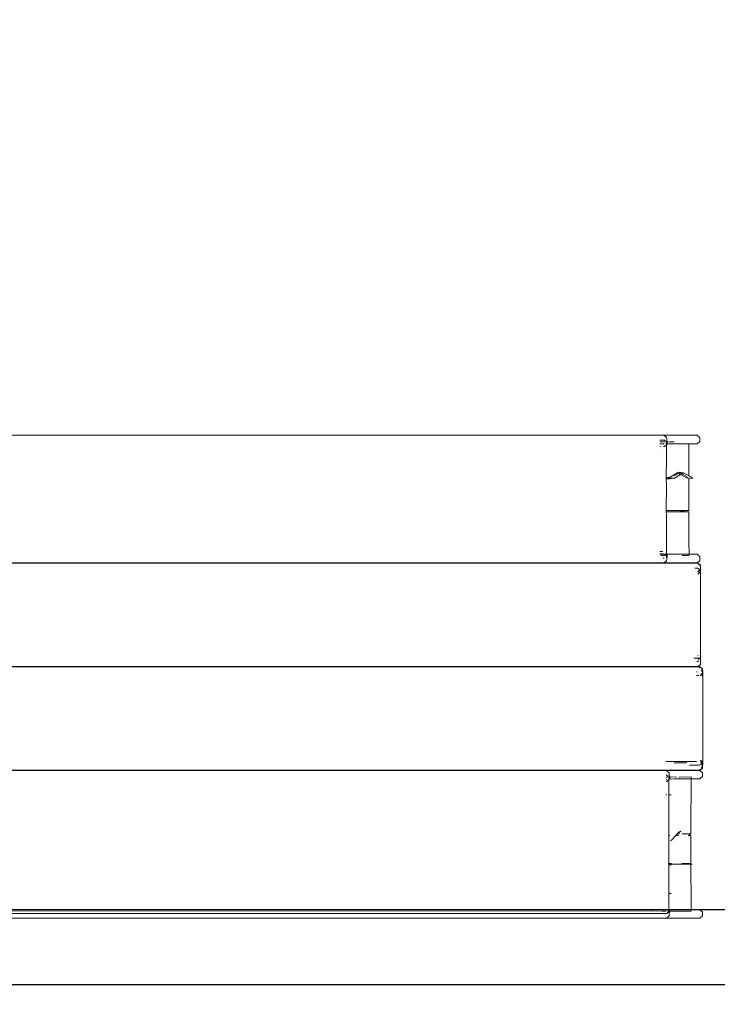
# Model space of a CAD drawing. Units: millimetres. Extents: x 7894 to 8038, y 6851 to 6951.
# Tile 4 of 49: x 7949.503 to 7954.151, y 6864.931 to 6871.489. Entities that reach past the tile are written whole.
import ezdxf

# ---------------------------------------------------------------- set-up
doc = ezdxf.new("R2010")
doc.units = ezdxf.units.MM
for name, color, linetype, lineweight in [('A-ANNO-DIMS', 2, 'Continuous', 18), ('A-FURN-BOOK', 8, 'Continuous', 13), ('A-FURN-CASE', 7, 'Continuous', 30)]:
    doc.layers.add(name, color=color, linetype=linetype, lineweight=lineweight)
doc.styles.get("Standard").update_dxf_attribs({"font": 'arial.ttf'})
doc.dimstyles.new('ISO-25', dxfattribs={"dimtxt": 1, "dimasz": 1, "dimexe": 1.25, "dimexo": 0.625, "dimtad": 1, "dimdec": 0, "dimlunit": 4, "dimtxsty": 'Standard', "dimcen": 2.5, "dimclrt": 1, "dimadec": 0, "dimazin": 0, "dimtfac": 1, "dimtdec": 0, "dimtmove": 0, "dimatfit": 3, "dimfxl": 1, "dimarcsym": 0})

# ---------------------------------------------------------------- blocks, each defined once
blk = doc.blocks.new('*D36')
at = {"layer": 'A-ANNO-DIMS', "color": 0, "lineweight": -2, "transparency": 16777216}
for p, q in [((7980.8359, 6877.9586), (7980.8359, 6858.5122)), ((7944.4866, 6864.4359), (7944.4866, 6858.5122)), ((7945.4866, 6859.7622), (7979.8359, 6859.7622))]:
    blk.add_line(p, q, dxfattribs=at)
at = {"layer": 'A-ANNO-DIMS', "color": 0, "transparency": 16777216}
for points in [[(7945.4866, 6859.9288), (7945.4866, 6859.5955), (7944.4866, 6859.7622)], [(7979.8359, 6859.9288), (7979.8359, 6859.5955), (7980.8359, 6859.7622)]]:
    blk.add_solid(points, dxfattribs=at)
at = {"layer": 'Defpoints', "color": 0, "transparency": 16777216}
for p in [(7980.8359, 6878.5836), (7944.4866, 6865.0609), (7980.8359, 6859.7622)]:
    blk.add_point(p, dxfattribs=at)
at = {"layer": 'A-ANNO-DIMS', "color": 1, "transparency": 16777216, "insert": (7962.6613, 6860.9046), "char_height": 1, "attachment_point": 5}
blk.add_mtext('3\'-0 1/2"', dxfattribs=at)
blk = doc.blocks.new('*D37')
at = {"layer": 'A-ANNO-DIMS', "color": 0, "lineweight": -2, "transparency": 16777216}
for p, q in [((7954.9197, 6887.9028), (7941.3891, 6887.9028)), ((7942.6391, 6862.6097), (7942.6391, 6886.9028)), ((7953.6228, 6861.6097), (7941.3891, 6861.6097))]:
    blk.add_line(p, q, dxfattribs=at)
at = {"layer": 'A-ANNO-DIMS', "color": 0, "transparency": 16777216}
for points in [[(7942.4724, 6886.9028), (7942.8057, 6886.9028), (7942.6391, 6887.9028)], [(7942.4724, 6862.6097), (7942.8057, 6862.6097), (7942.6391, 6861.6097)]]:
    blk.add_solid(points, dxfattribs=at)
at = {"layer": 'Defpoints', "color": 0, "transparency": 16777216}
for p in [(7942.6391, 6887.9028), (7955.5447, 6887.9028), (7954.2478, 6861.6097)]:
    blk.add_point(p, dxfattribs=at)
at = {"layer": 'A-ANNO-DIMS', "color": 1, "transparency": 16777216, "insert": (7941.497, 6874.7562), "char_height": 1, "attachment_point": 5, "rotation": 90}
blk.add_mtext('2\'-2 1/2"', dxfattribs=at)

msp = doc.modelspace()

# ---------------------------------------------------------------- linework, layer by layer
at = {"layer": 'A-FURN-BOOK'}
for p, q in [((7953.7957, 6868.7211), (7945.1072, 6868.7211)), ((7953.7988, 6868.6885), (7953.7677, 6868.6885)), ((7953.8027, 6868.7151), (7953.7957, 6868.7211)), ((7954.0176, 6868.7211), (7953.7957, 6868.7211)), ((7953.8072, 6868.6808), (7953.7988, 6868.6885)), ((7953.8027, 6868.7151), (7953.8123, 6868.7081)), ((7953.8123, 6868.7069), (7953.8123, 6868.7081)), ((7953.8133, 6868.706), (7953.8123, 6868.7069)), ((7953.8131, 6868.677), (7953.8143, 6868.693)), ((7953.8143, 6868.693), (7953.8133, 6868.706)), ((7953.8158, 6868.6777), (7953.8143, 6868.693)), ((7954.0176, 6868.7211), (7954.0351, 6868.705)), ((7954.0351, 6868.705), (7954.0351, 6868.6797)), ((7953.7697, 6868.6769), (7953.7676, 6868.6775)), ((7953.7676, 6868.6636), (7953.7935, 6868.6636)), ((7953.7721, 6868.6458), (7953.7676, 6868.6458)), ((7953.8046, 6868.6775), (7953.7697, 6868.6769)), ((7953.7961, 6868.6612), (7953.7935, 6868.6612)), ((7953.7988, 6868.6458), (7953.7935, 6868.6458)), ((7953.7973, 6868.6621), (7953.7961, 6868.6612)), ((7953.8126, 6868.6585), (7953.7988, 6868.6458)), ((7953.8114, 6868.6769), (7953.8131, 6868.677)), ((7953.8132, 6868.6753), (7953.8114, 6868.6769)), ((7953.8132, 6868.6742), (7953.8114, 6868.6729)), ((7953.8114, 6868.6636), (7953.8132, 6868.6742)), ((7953.8126, 6868.6618), (7953.8114, 6868.6636)), ((7953.8127, 6868.6636), (7953.8114, 6868.6636)), ((7953.8124, 6868.5618), (7953.8125, 6868.6434)), ((7953.8125, 6868.6434), (7953.8126, 6868.6585)), ((7953.8163, 6868.6619), (7953.8126, 6868.6585)), ((7953.8126, 6868.6585), (7953.8126, 6868.6618)), ((7953.8168, 6868.6626), (7953.8127, 6868.6636)), ((7953.8131, 6868.677), (7953.8158, 6868.6777)), ((7953.8132, 6868.6753), (7953.8131, 6868.677)), ((7953.8163, 6868.6724), (7953.8132, 6868.6753)), ((7953.8132, 6868.6742), (7953.8132, 6868.6753)), ((7953.8192, 6868.6797), (7953.8158, 6868.6777)), ((7953.8158, 6868.6777), (7953.8187, 6868.6773)), ((7953.8163, 6868.6724), (7953.8158, 6868.6777)), ((7953.8163, 6868.6619), (7953.8168, 6868.6626)), ((7953.8168, 6868.6626), (7953.8172, 6868.6668)), ((7953.8168, 6868.6626), (7953.823, 6868.6636)), ((7953.8172, 6868.6668), (7953.8182, 6868.6753)), ((7953.8182, 6868.6753), (7953.8187, 6868.6773)), ((7953.8187, 6868.6773), (7953.8192, 6868.6797)), ((7953.8187, 6868.6773), (7953.8224, 6868.6775)), ((7953.823, 6868.6636), (7953.9622, 6868.6636)), ((7953.8317, 6868.6771), (7953.828, 6868.6775)), ((7953.8639, 6868.6775), (7953.8317, 6868.6771)), ((7953.9622, 6868.6636), (7953.9615, 6868.5883)), ((7953.9622, 6868.6636), (7954.0176, 6868.6636)), ((7954.0351, 6868.6797), (7954.0176, 6868.6636)), ((7953.769, 6868.5883), (7953.7676, 6868.5883)), ((7953.8113, 6868.4406), (7953.8124, 6868.5618)), ((7953.9615, 6868.5883), (7953.9608, 6868.4903)), ((7953.9608, 6868.4903), (7953.9607, 6868.4519)), ((7953.8123, 6868.4394), (7953.8113, 6868.4406)), ((7953.8113, 6868.4394), (7953.8113, 6868.4406)), ((7953.8113, 6868.4394), (7953.8123, 6868.4394)), ((7953.8113, 6868.4363), (7953.8113, 6868.4394)), ((7953.8113, 6868.4363), (7953.8123, 6868.4363)), ((7953.8113, 6868.4348), (7953.8113, 6868.4363)), ((7953.8113, 6868.4348), (7953.8373, 6868.435)), ((7953.8113, 6868.432), (7953.8113, 6868.4348)), ((7953.8113, 6868.432), (7953.8123, 6868.4308)), ((7953.8113, 6868.4308), (7953.8113, 6868.432)), ((7953.8123, 6868.4308), (7953.8113, 6868.4308)), ((7953.8123, 6868.3879), (7953.8113, 6868.4308)), ((7953.8289, 6868.4406), (7953.8123, 6868.4394)), ((7953.8123, 6868.4363), (7953.8373, 6868.435)), ((7953.8302, 6868.4309), (7953.8123, 6868.4308)), ((7953.8289, 6868.4406), (7953.8302, 6868.4395)), ((7953.8302, 6868.4395), (7953.832, 6868.4406)), ((7953.8321, 6868.432), (7953.8302, 6868.4309)), ((7953.8334, 6868.4406), (7953.832, 6868.4406)), ((7953.8651, 6868.4352), (7953.8321, 6868.432)), ((7953.8373, 6868.435), (7953.8321, 6868.432)), ((7953.8334, 6868.4406), (7953.8922, 6868.4752)), ((7953.8373, 6868.435), (7953.8384, 6868.4363)), ((7953.8651, 6868.4352), (7953.8384, 6868.4363)), ((7953.8922, 6868.4666), (7953.8644, 6868.4506)), ((7953.8651, 6868.4352), (7953.9068, 6868.4592)), ((7953.927, 6868.4709), (7953.8922, 6868.4752)), ((7953.8922, 6868.4752), (7953.9059, 6868.4683)), ((7953.9059, 6868.4683), (7953.8922, 6868.4666)), ((7953.9006, 6868.4623), (7953.8922, 6868.4666)), ((7953.927, 6868.4709), (7953.9059, 6868.4683)), ((7953.9059, 6868.4683), (7953.911, 6868.4657)), ((7953.9068, 6868.4592), (7953.9147, 6868.4638)), ((7953.9437, 6868.4406), (7953.9068, 6868.4592)), ((7953.9147, 6868.4638), (7953.927, 6868.4709)), ((7953.9147, 6868.4638), (7953.9475, 6868.4472)), ((7953.9607, 6868.4519), (7953.927, 6868.4709)), ((7953.9533, 6868.4406), (7953.9437, 6868.4406)), ((7953.9522, 6868.4363), (7953.9437, 6868.4406)), ((7953.9522, 6868.4363), (7953.957, 6868.4363)), ((7953.9607, 6868.432), (7953.9522, 6868.4363)), ((7953.9607, 6868.432), (7953.9605, 6868.3823)), ((7953.9884, 6868.4363), (7953.9607, 6868.4519)), ((7953.9884, 6868.4363), (7953.9607, 6868.432)), ((7953.8113, 6868.2194), (7953.8123, 6868.3879)), ((7953.9605, 6868.2194), (7953.9605, 6868.3823)), ((7953.8113, 6868.2194), (7953.8301, 6868.2195)), ((7953.8113, 6868.2109), (7953.8113, 6868.2194)), ((7953.8123, 6868.1936), (7953.8113, 6868.2109)), ((7953.8123, 6868.2109), (7953.8113, 6868.2109)), ((7953.8123, 6868.2109), (7953.8301, 6868.2109)), ((7953.8123, 6868.1936), (7953.8125, 6867.9487)), ((7953.8301, 6868.2195), (7953.9605, 6868.2194)), ((7953.8301, 6868.2109), (7953.9605, 6868.2109)), ((7953.9605, 6868.2194), (7953.905, 6868.2151)), ((7953.905, 6868.2151), (7953.9605, 6868.2109)), ((7953.9608, 6868.1072), (7953.9605, 6868.2109)), ((7953.9608, 6868.1072), (7953.9615, 6868.0092)), ((7953.7675, 6868.0092), (7953.769, 6868.0092)), ((7953.9615, 6868.0092), (7953.9635, 6867.9285)), ((7953.7889, 6867.9463), (7953.7676, 6867.9463)), ((7953.7939, 6867.9309), (7953.7676, 6867.9309)), ((7953.7676, 6867.9285), (7953.7993, 6867.9285)), ((7953.774, 6867.9205), (7953.8044, 6867.9199)), ((7953.8044, 6867.9199), (7953.7745, 6867.9199)), ((7953.7969, 6867.9036), (7953.7876, 6867.9036)), ((7953.7993, 6867.9285), (7953.7973, 6867.93)), ((7953.8018, 6867.9285), (7953.7993, 6867.9285)), ((7953.8018, 6867.9285), (7953.8064, 6867.9243)), ((7953.806, 6867.9234), (7953.8018, 6867.9285)), ((7953.8083, 6867.9285), (7953.8018, 6867.9285)), ((7953.8126, 6867.9336), (7953.8109, 6867.9351)), ((7953.8114, 6867.9285), (7953.8126, 6867.9303)), ((7953.8127, 6867.9285), (7953.8114, 6867.9285)), ((7953.8114, 6867.9204), (7953.8114, 6867.9285)), ((7953.8114, 6867.9204), (7953.8131, 6867.9196)), ((7953.8131, 6867.9196), (7953.8114, 6867.9196)), ((7953.8132, 6867.9168), (7953.8114, 6867.9152)), ((7953.8126, 6867.9336), (7953.8125, 6867.9487)), ((7953.8126, 6867.9303), (7953.8126, 6867.9336)), ((7953.8163, 6867.9302), (7953.8126, 6867.9336)), ((7953.8168, 6867.9295), (7953.8127, 6867.9285)), ((7953.8163, 6867.9197), (7953.8131, 6867.9196)), ((7953.8132, 6867.9179), (7953.8131, 6867.9196)), ((7953.8163, 6867.9197), (7953.8132, 6867.9179)), ((7953.8132, 6867.9179), (7953.8132, 6867.9168)), ((7953.8132, 6867.9168), (7953.8143, 6867.898)), ((7953.8132, 6867.9168), (7953.8158, 6867.9148)), ((7953.8134, 6867.8858), (7953.8143, 6867.898)), ((7953.8143, 6867.898), (7953.8158, 6867.9148)), ((7953.8158, 6867.9148), (7953.8163, 6867.9197)), ((7953.8158, 6867.9148), (7953.8192, 6867.9124)), ((7953.8168, 6867.9295), (7953.8163, 6867.9302)), ((7953.823, 6867.9285), (7953.8168, 6867.9295)), ((7953.8173, 6867.9251), (7953.8168, 6867.9295)), ((7953.8182, 6867.9168), (7953.8173, 6867.9251)), ((7953.8192, 6867.9124), (7953.8182, 6867.9168)), ((7953.9635, 6867.9285), (7953.823, 6867.9285)), ((7953.9181, 6867.92), (7953.9193, 6867.9199)), ((7953.9623, 6867.9199), (7953.9193, 6867.9199)), ((7953.9635, 6867.9285), (7953.9623, 6867.9199)), ((7953.9635, 6867.9285), (7954.0176, 6867.9285)), ((7954.0176, 6867.9285), (7954.0351, 6867.9124)), ((7954.0351, 6867.9124), (7954.0351, 6867.8871)), ((7953.7957, 6867.871), (7945.1072, 6867.871)), ((7954.0211, 6867.8683), (7945.3118, 6867.8683)), ((7953.7957, 6867.871), (7953.8123, 6867.884)), ((7953.7957, 6867.871), (7954.0176, 6867.871)), ((7953.8123, 6867.884), (7953.8134, 6867.8858)), ((7954.0211, 6867.8366), (7954.0011, 6867.8366)), ((7954.0351, 6867.8871), (7954.0176, 6867.871)), ((7954.0211, 6867.8683), (7954.0386, 6867.8526)), ((7954.0386, 6867.8535), (7954.0211, 6867.8683)), ((7954.0211, 6867.8683), (7954.0386, 6867.8556)), ((7954.0343, 6867.8246), (7954.0211, 6867.8366)), ((7954.0386, 6867.8535), (7954.0386, 6867.8556)), ((7954.0386, 6867.8526), (7954.0386, 6867.8535)), ((7954.0386, 6867.8287), (7954.0386, 6867.8526)), ((7954.0343, 6867.8246), (7954.0211, 6867.8123)), ((7954.0375, 6867.8217), (7954.0211, 6867.81)), ((7954.0386, 6867.8106), (7954.0211, 6867.795)), ((7954.0386, 6867.8287), (7954.0343, 6867.8246)), ((7954.0375, 6867.8217), (7954.0343, 6867.8246)), ((7954.0375, 6867.8217), (7954.0386, 6867.8237)), ((7954.0386, 6867.8224), (7954.0375, 6867.8217)), ((7954.0386, 6867.8207), (7954.0375, 6867.8217)), ((7954.0386, 6867.8237), (7954.0386, 6867.8287)), ((7954.0386, 6867.8237), (7954.0386, 6867.8224)), ((7954.0386, 6867.8224), (7954.0386, 6867.8207)), ((7954.0386, 6867.8216), (7954.0386, 6867.8224)), ((7954.0386, 6867.8207), (7954.0386, 6867.8216)), ((7954.0386, 6867.8106), (7954.0386, 6867.8207)), ((7954.0386, 6867.8106), (7954.0386, 6867.1943)), ((7954.024, 6867.2523), (7954.0211, 6867.2549)), ((7954.037, 6867.2407), (7954.0347, 6867.2427)), ((7954.0211, 6867.1816), (7945.1072, 6867.1816)), ((7945.1072, 6867.1782), (7954.0292, 6867.1782)), ((7953.9953, 6867.2376), (7954.0211, 6867.2376)), ((7954.0211, 6867.2133), (7954.0153, 6867.2133)), ((7954.0211, 6867.2376), (7954.0313, 6867.2284)), ((7954.0267, 6867.2183), (7954.0211, 6867.2133)), ((7954.0386, 6867.1943), (7954.0211, 6867.1816)), ((7954.0327, 6867.2315), (7954.0232, 6867.2384)), ((7954.0292, 6867.1782), (7954.0368, 6867.1714)), ((7954.0365, 6867.1782), (7954.0292, 6867.1782)), ((7954.0365, 6867.1782), (7954.0536, 6867.1655)), ((7954.0176, 6867.1465), (7954.0117, 6867.1465)), ((7954.0292, 6867.1222), (7954.0118, 6867.1222)), ((7954.0393, 6867.1216), (7954.038, 6867.1221)), ((7954.0393, 6867.1216), (7954.0496, 6867.1308)), ((7954.0491, 6867.1319), (7954.0464, 6867.1336)), ((7954.0469, 6867.1606), (7954.0476, 6867.1555)), ((7954.0496, 6867.1205), (7954.0473, 6867.1184)), ((7954.0476, 6867.1555), (7954.0481, 6867.1476)), ((7954.0488, 6867.1367), (7954.0491, 6867.1319)), ((7954.0491, 6867.1319), (7954.0496, 6867.1308)), ((7954.0496, 6867.1308), (7954.0515, 6867.1306)), ((7954.0501, 6867.1234), (7954.0496, 6867.1205)), ((7954.0515, 6867.1306), (7954.0501, 6867.1234)), ((7954.0521, 6867.1323), (7954.0515, 6867.1306)), ((7954.0521, 6867.1323), (7954.053, 6867.1421)), ((7954.053, 6867.1449), (7954.0536, 6867.1655)), ((7954.0536, 6867.1655), (7954.0545, 6867.1441)), ((7954.0545, 6867.1441), (7954.0549, 6867.0366)), ((7954.0549, 6867.0366), (7954.0551, 6866.9067)), ((7954.0551, 6866.9067), (7954.0551, 6866.7576)), ((7954.0551, 6866.7576), (7954.0546, 6866.5541)), ((7953.9438, 6866.5475), (7953.8077, 6866.5475)), ((7953.9437, 6866.5393), (7953.8633, 6866.5389)), ((7953.9438, 6866.5475), (7953.9437, 6866.5393)), ((7954.0119, 6866.5475), (7953.9438, 6866.5475)), ((7954.0317, 6866.5232), (7953.9654, 6866.5232)), ((7954.0496, 6866.5389), (7954.0376, 6866.5479)), ((7954.0491, 6866.5378), (7954.0376, 6866.5281)), ((7954.0496, 6866.5492), (7954.0397, 6866.558)), ((7954.0486, 6866.5301), (7954.0481, 6866.5221)), ((7954.0491, 6866.5378), (7954.0486, 6866.5301)), ((7954.0496, 6866.5389), (7954.0491, 6866.5378)), ((7954.0496, 6866.5492), (7954.0501, 6866.5463)), ((7954.052, 6866.5386), (7954.0496, 6866.5389)), ((7954.0501, 6866.5463), (7954.0514, 6866.5403)), ((7954.0514, 6866.5403), (7954.052, 6866.5386)), ((7954.052, 6866.5386), (7954.0527, 6866.5371)), ((7954.0527, 6866.5371), (7954.053, 6866.5248)), ((7954.0545, 6866.5256), (7954.053, 6866.5248)), ((7954.0536, 6866.5042), (7954.053, 6866.5248)), ((7954.0546, 6866.5541), (7954.0545, 6866.5256)), ((7945.1072, 6866.4885), (7953.8124, 6866.4885)), ((7954.0365, 6866.4915), (7945.8962, 6866.4915)), ((7953.8156, 6866.4567), (7953.8102, 6866.4567)), ((7953.8195, 6866.4826), (7953.8124, 6866.4885)), ((7953.8124, 6866.4885), (7954.0343, 6866.4885)), ((7953.8239, 6866.4492), (7953.8156, 6866.4567)), ((7953.8282, 6866.4753), (7953.8195, 6866.4826)), ((7953.8195, 6866.4826), (7953.829, 6866.4758)), ((7953.8289, 6866.4746), (7953.829, 6866.4758)), ((7953.83, 6866.4737), (7953.8289, 6866.4746)), ((7953.83, 6866.4737), (7953.829, 6866.4758)), ((7953.8298, 6866.4454), (7953.8311, 6866.461)), ((7953.8311, 6866.461), (7953.83, 6866.4737)), ((7953.8325, 6866.4462), (7953.8311, 6866.461)), ((7954.0368, 6866.4983), (7954.0331, 6866.4949)), ((7954.0343, 6866.4885), (7954.0518, 6866.4728)), ((7954.0536, 6866.5042), (7954.0365, 6866.4915)), ((7954.0467, 6866.5072), (7954.0431, 6866.504)), ((7954.0474, 6866.5121), (7954.0467, 6866.5072)), ((7954.0518, 6866.4728), (7954.0518, 6866.4481)), ((7953.8128, 6866.4301), (7953.8101, 6866.4301)), ((7953.8156, 6866.4151), (7953.8101, 6866.4151)), ((7953.8203, 6866.4449), (7953.8102, 6866.4448)), ((7953.814, 6866.431), (7953.8128, 6866.4301)), ((7953.8293, 6866.4275), (7953.8156, 6866.4151)), ((7953.8278, 6866.326), (7953.8291, 6866.4128)), ((7953.8299, 6866.4439), (7953.8281, 6866.4454)), ((7953.8298, 6866.4454), (7953.8281, 6866.4454)), ((7953.8299, 6866.4428), (7953.8281, 6866.4415)), ((7953.8281, 6866.4325), (7953.8299, 6866.4428)), ((7953.8293, 6866.4308), (7953.8281, 6866.4325)), ((7953.8294, 6866.4325), (7953.8281, 6866.4325)), ((7953.8291, 6866.4128), (7953.8293, 6866.4275)), ((7953.8293, 6866.4275), (7953.8293, 6866.4308)), ((7953.833, 6866.4308), (7953.8293, 6866.4275)), ((7953.8335, 6866.4315), (7953.8294, 6866.4325)), ((7953.8325, 6866.4462), (7953.8298, 6866.4454)), ((7953.8298, 6866.4454), (7953.8299, 6866.4439)), ((7953.833, 6866.441), (7953.8299, 6866.4439)), ((7953.8299, 6866.4428), (7953.8299, 6866.4439)), ((7953.8359, 6866.4481), (7953.8325, 6866.4462)), ((7953.8353, 6866.4454), (7953.8325, 6866.4462)), ((7953.833, 6866.441), (7953.8325, 6866.4462)), ((7953.833, 6866.4308), (7953.8335, 6866.4315)), ((7953.8335, 6866.4315), (7953.8339, 6866.4356)), ((7953.8656, 6866.4325), (7953.8335, 6866.4315)), ((7953.8339, 6866.4356), (7953.8349, 6866.4439)), ((7953.8349, 6866.4439), (7953.8353, 6866.4454)), ((7953.8353, 6866.4454), (7953.8359, 6866.4481)), ((7953.8469, 6866.4449), (7953.8353, 6866.4454)), ((7953.8799, 6866.4454), (7953.8469, 6866.4449)), ((7953.9773, 6866.4325), (7953.8656, 6866.4325)), ((7953.9003, 6866.4454), (7953.9018, 6866.4451)), ((7953.9774, 6866.4454), (7953.9018, 6866.4451)), ((7953.9773, 6866.4325), (7953.9766, 6866.326)), ((7953.9774, 6866.4454), (7953.9773, 6866.4325)), ((7953.9773, 6866.4325), (7954.0343, 6866.4325)), ((7954.0518, 6866.4481), (7954.0343, 6866.4325)), ((7953.8143, 6866.326), (7953.8098, 6866.326)), ((7953.8287, 6866.2927), (7953.8278, 6866.326)), ((7953.8444, 6866.326), (7953.8278, 6866.326)), ((7953.9766, 6866.326), (7953.9759, 6866.1997)), ((7953.8285, 6866.099), (7953.8287, 6866.2927)), ((7953.9756, 6866.066), (7953.9759, 6866.1997)), ((7953.8275, 6866.066), (7953.8285, 6866.099)), ((7953.8275, 6866.0549), (7953.8275, 6866.066)), ((7953.8275, 6866.066), (7953.8315, 6866.066)), ((7953.8871, 6866.066), (7953.8739, 6866.0549)), ((7953.8739, 6866.0549), (7953.8847, 6866.066)), ((7953.8813, 6866.066), (7953.8847, 6866.066)), ((7953.8847, 6866.066), (7953.8981, 6866.0798)), ((7953.9072, 6866.0853), (7953.8871, 6866.066)), ((7953.8871, 6866.066), (7953.8987, 6866.066)), ((7953.9072, 6866.0853), (7953.8981, 6866.0798)), ((7953.9173, 6866.066), (7953.9756, 6866.066)), ((7953.9756, 6866.066), (7953.9636, 6866.0605)), ((7953.9636, 6866.0605), (7953.9756, 6866.0549)), ((7953.8285, 6865.8767), (7953.8275, 6866.0549)), ((7953.8358, 6866.0549), (7953.8275, 6866.0549)), ((7953.8392, 6866.0193), (7953.8452, 6866.0248)), ((7953.8739, 6866.0549), (7953.8452, 6866.0248)), ((7953.8739, 6866.0549), (7953.87, 6866.0549)), ((7953.8873, 6866.0549), (7953.8782, 6866.0549)), ((7953.8929, 6866.0549), (7953.8915, 6866.0549)), ((7953.9756, 6866.0549), (7953.9564, 6866.0549)), ((7953.9756, 6865.9341), (7953.9756, 6866.0549)), ((7953.9756, 6865.9341), (7953.9758, 6865.87)), ((7953.8269, 6865.87), (7953.8285, 6865.8767)), ((7953.8275, 6865.8645), (7953.8269, 6865.87)), ((7953.8453, 6865.87), (7953.8269, 6865.87)), ((7953.8276, 6865.859), (7953.8275, 6865.8645)), ((7953.9836, 6865.8645), (7953.8275, 6865.8645)), ((7953.9758, 6865.87), (7953.9158, 6865.87)), ((7953.9758, 6865.87), (7953.9836, 6865.8645)), ((7953.9758, 6865.859), (7953.9836, 6865.8645)), ((7953.8287, 6865.6968), (7953.8276, 6865.859)), ((7953.8276, 6865.859), (7953.844, 6865.859)), ((7953.9759, 6865.7949), (7953.9758, 6865.859)), ((7953.9759, 6865.7949), (7953.9766, 6865.6686)), ((7953.8278, 6865.6686), (7953.8287, 6865.6968)), ((7953.8291, 6865.5806), (7953.8278, 6865.6686)), ((7953.8278, 6865.6686), (7953.8444, 6865.6686)), ((7953.9766, 6865.6686), (7953.9774, 6865.5609)), ((7953.7178, 6865.5609), (7945.1072, 6865.5609)), ((7953.7178, 6865.5527), (7945.1072, 6865.5519)), ((7953.8102, 6865.5367), (7945.1072, 6865.5367)), ((7953.7178, 6865.5609), (7953.7178, 6865.5527)), ((7953.8101, 6865.5609), (7953.7178, 6865.5609)), ((7953.7178, 6865.5527), (7953.7848, 6865.5525)), ((7953.7848, 6865.5525), (7953.8101, 6865.5519)), ((7953.8156, 6865.5367), (7953.8136, 6865.5367)), ((7953.8299, 6865.5506), (7953.8156, 6865.5367)), ((7953.8207, 6865.5519), (7953.8285, 6865.5519)), ((7953.8285, 6865.5519), (7953.8226, 6865.556)), ((7953.823, 6865.5568), (7953.8285, 6865.5519)), ((7953.8294, 6865.5609), (7953.825, 6865.5609)), ((7953.8293, 6865.5659), (7953.8279, 6865.5672)), ((7953.8285, 6865.5519), (7953.8294, 6865.5609)), ((7953.8299, 6865.5506), (7953.8285, 6865.5519)), ((7953.8293, 6865.5659), (7953.8291, 6865.5806)), ((7953.8293, 6865.5626), (7953.8293, 6865.5659)), ((7953.833, 6865.5626), (7953.8293, 6865.5659)), ((7953.8294, 6865.5609), (7953.8293, 6865.5626)), ((7953.8335, 6865.5619), (7953.8294, 6865.5609)), ((7953.833, 6865.5523), (7953.8299, 6865.5506)), ((7953.8299, 6865.5506), (7953.8299, 6865.5495)), ((7953.8299, 6865.5506), (7953.8325, 6865.5476)), ((7953.8349, 6865.5495), (7953.8299, 6865.5506)), ((7953.8299, 6865.5495), (7953.831, 6865.5312)), ((7953.831, 6865.5312), (7953.8325, 6865.5476)), ((7953.8325, 6865.5476), (7953.833, 6865.5523)), ((7953.8325, 6865.5476), (7953.8359, 6865.5452)), ((7953.8335, 6865.5619), (7953.833, 6865.5626)), ((7953.833, 6865.5523), (7953.8346, 6865.5519)), ((7953.8656, 6865.5609), (7953.8335, 6865.5619)), ((7953.834, 6865.5576), (7953.8335, 6865.5619)), ((7953.8346, 6865.5519), (7953.834, 6865.5576)), ((7953.8346, 6865.5519), (7953.8469, 6865.5523)), ((7953.8349, 6865.5495), (7953.8346, 6865.5519)), ((7953.9088, 6865.5521), (7953.8349, 6865.5495)), ((7953.8359, 6865.5452), (7953.8349, 6865.5495)), ((7953.8469, 6865.5523), (7953.9088, 6865.5521)), ((7953.8656, 6865.5609), (7953.9774, 6865.5609)), ((7953.9088, 6865.5521), (7953.9774, 6865.5519)), ((7953.9774, 6865.5609), (7953.9774, 6865.5519)), ((7953.9774, 6865.5609), (7954.0343, 6865.5609)), ((7954.0343, 6865.5609), (7954.0518, 6865.5452)), ((7954.0518, 6865.5452), (7954.0518, 6865.5206)), ((7953.8124, 6865.5049), (7945.1072, 6865.5049)), ((7953.8124, 6865.5049), (7953.829, 6865.5176)), ((7953.8124, 6865.5049), (7954.0343, 6865.5049)), ((7953.829, 6865.5176), (7953.8301, 6865.5194)), ((7953.8301, 6865.5194), (7953.831, 6865.5312)), ((7954.0518, 6865.5206), (7954.0343, 6865.5049))]:
    msp.add_line(p, q, dxfattribs=at)
at = {"layer": 'A-FURN-CASE'}
for points in [[(7944.4866, 6876.4609), (7955.8866, 6876.4609), (7955.8866, 6865.0609), (7944.4866, 6865.0609)], [(7944.9866, 6875.9609), (7955.3866, 6875.9609), (7955.3866, 6865.5609), (7944.9866, 6865.5609)]]:
    msp.add_lwpolyline(points, close=True, dxfattribs=at)

# ---------------------------------------------------------------- dimensions: what is measured, and where the dimension line sits
at = {"layer": 'A-ANNO-DIMS'}
dim = msp.add_linear_dim(base=(7942.6391, 6887.9028), p1=(7954.2478, 6861.6097), p2=(7955.5447, 6887.9028), angle=90, dimstyle='ISO-25', override={"dimdec": 1, "dimlfac": 1, "dimrnd": 0, "dimzin": 1, "dimdsep": 46, "dimlunit": 4, "dimfrac": 2}, dxfattribs=at)
dim.commit()
dim.dimension.update_dxf_attribs({"geometry": '*D37', "text_midpoint": (7941.497, 6874.7562)})
dim = msp.add_linear_dim(base=(7980.8359, 6859.7622), p1=(7944.4866, 6865.0609), p2=(7980.8359, 6878.5836), dimstyle='ISO-25', override={"dimdec": 1, "dimlfac": 1, "dimrnd": 0, "dimzin": 1, "dimdsep": 46, "dimlunit": 4, "dimfrac": 2}, dxfattribs=at)
dim.commit()
dim.dimension.update_dxf_attribs({"geometry": '*D36', "text_midpoint": (7962.6613, 6860.9046)})

doc.saveas('drawing.dxf')
